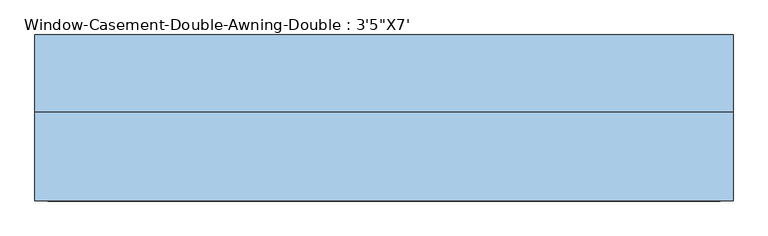
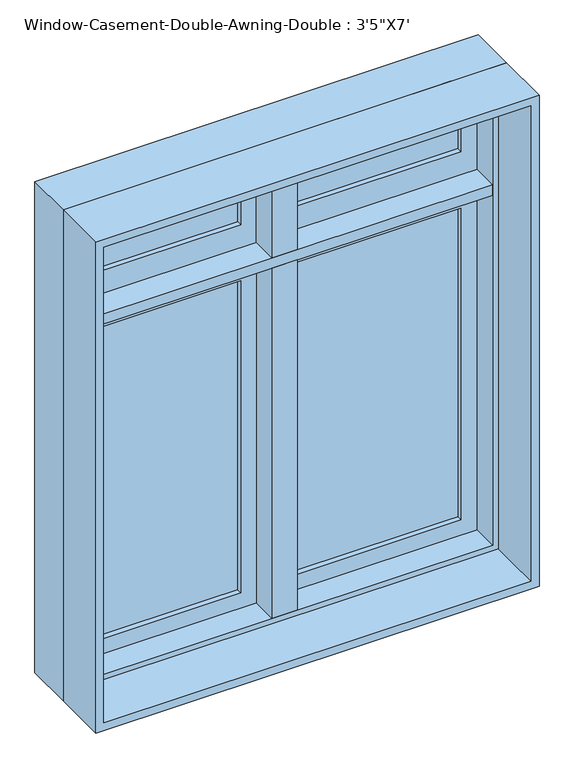
"""IFC4 building model written with IfcOpenShell, lengths in millimetres: window geometry."""

from ifc_helpers import new_model, si_unit, frame, origin, place, context, project, spatial, polyline, outline, extrude, faceted_brep, source, transform, mapped, element, save


def window_35f3c129(model_context):
    return source(origin(), model_context, "Body", "SolidModel", [
        faceted_brep([(488.95, 82.55, 2101.85), (488.95, 19.05, 2101.85), (-488.95, 19.05, 2101.85), (-488.95, 82.55, 2101.85), (508.0, 133.35, 2120.9), (508.0, 82.55, 2120.9), (-508.0, 82.55, 2120.9), (-508.0, 133.35, 2120.9), (520.7, 19.05, 2133.6), (520.7, 133.35, 2133.6), (-520.7, 133.35, 2133.6), (-520.7, 19.05, 2133.6), (-488.95, 19.05, 946.15), (-488.95, 82.55, 946.15), (-508.0, 82.55, 927.1), (-508.0, 133.35, 927.1), (-520.7, 133.35, 914.4), (-520.7, 19.05, 914.4), (488.95, 19.05, 946.15), (488.95, 82.55, 946.15), (508.0, 82.55, 927.1), (508.0, 133.35, 927.1), (520.7, 133.35, 914.4), (520.7, 19.05, 914.4)], [[[0, 1, 2, 3]], [[4, 5, 6, 7]], [[8, 9, 10, 11]], [[3, 2, 12, 13]], [[7, 6, 14, 15]], [[11, 10, 16, 17]], [[13, 12, 18, 19]], [[15, 14, 20, 21]], [[17, 16, 22, 23]], [[11, 17, 23, 8], [1, 18, 12, 2]], [[19, 18, 1, 0]], [[5, 20, 14, 6], [3, 13, 19, 0]], [[21, 20, 5, 4]], [[23, 22, 9, 8]], [[9, 22, 16, 10], [7, 15, 21, 4]]]),
        extrude(outline(polyline([(2133.6, -520.7), (914.4, -520.7), (914.4, 520.7), (2133.6, 520.7), (2133.6, -520.7)]), holes=[polyline([(2114.55, 501.65), (933.45, 501.65), (933.45, -501.65), (2114.55, -501.65), (2114.55, 501.65)])]), frame((0.0, -114.3, 0.0), z_axis=(0.0, 1.0, 0.0), x_axis=(0.0, 0.0, 1.0)), (0.0, 0.0, 1.0), 133.35),
        extrude(outline(polyline([(927.1, 508.0), (1816.1, 508.0), (1816.1, 9.525), (927.1, 9.525), (927.1, 508.0)]), holes=[polyline([(984.25, 66.675), (1758.95, 66.675), (1758.95, 450.85), (984.25, 450.85), (984.25, 66.675)])]), frame((0.0, 82.55, 0.0), z_axis=(0.0, 1.0, 0.0), x_axis=(0.0, 0.0, 1.0)), (0.0, 0.0, 1.0), 44.45),
        extrude(outline(polyline([(1816.1, -508.0), (927.1, -508.0), (927.1, -9.525), (1816.1, -9.525), (1816.1, -508.0)]), holes=[polyline([(1758.95, -66.675), (984.25, -66.675), (984.25, -450.85), (1758.95, -450.85), (1758.95, -66.675)])]), frame((0.0, 82.55, 0.0), z_axis=(0.0, 1.0, 0.0), x_axis=(0.0, 0.0, 1.0)), (0.0, 0.0, 1.0), 44.45),
        extrude(outline(polyline([(450.85, 114.3), (450.85, 107.95), (66.675, 107.95), (66.675, 114.3), (450.85, 114.3)])), frame((0.0, 0.0, 984.25), z_axis=(0.0, 0.0, 1.0), x_axis=(1.0, 0.0, 0.0)), (0.0, 0.0, 1.0), 774.7),
        extrude(outline(polyline([(66.675, 95.25), (66.675, 101.6), (450.85, 101.6), (450.85, 95.25), (66.675, 95.25)])), frame((0.0, 0.0, 984.25), z_axis=(0.0, 0.0, 1.0), x_axis=(1.0, 0.0, 0.0)), (0.0, 0.0, 1.0), 774.7),
        extrude(outline(polyline([(-66.675, 114.3), (-66.675, 107.95), (-450.85, 107.95), (-450.85, 114.3), (-66.675, 114.3)])), frame((0.0, 0.0, 984.25), z_axis=(0.0, 0.0, 1.0), x_axis=(1.0, 0.0, 0.0)), (0.0, 0.0, 1.0), 774.7),
        extrude(outline(polyline([(-450.85, 95.25), (-450.85, 101.6), (-66.675, 101.6), (-66.675, 95.25), (-450.85, 95.25)])), frame((0.0, 0.0, 984.25), z_axis=(0.0, 0.0, 1.0), x_axis=(1.0, 0.0, 0.0)), (0.0, 0.0, 1.0), 774.7),
        faceted_brep([(9.525, 133.35, 1816.1), (-9.525, 133.35, 1816.1), (-9.525, 82.55, 1816.1), (-30.1625, 82.55, 1816.1), (-30.1625, 19.05, 1816.1), (30.1625, 19.05, 1816.1), (30.1625, 82.55, 1816.1), (9.525, 82.55, 1816.1), (9.525, 133.35, 927.1), (9.525, 82.55, 927.1), (-9.525, 82.55, 927.1), (-9.525, 133.35, 927.1), (-9.525, 82.55, 946.15), (-30.1625, 82.55, 946.15), (-30.1625, 19.05, 946.15), (30.1625, 19.05, 946.15), (30.1625, 82.55, 946.15), (9.525, 82.55, 946.15)], [[[0, 1, 2, 3, 4, 5, 6, 7]], [[8, 9, 10, 11]], [[1, 0, 8, 11]], [[2, 1, 11, 10, 12]], [[3, 2, 12, 13]], [[4, 3, 13, 14]], [[5, 4, 14, 15]], [[6, 5, 15, 16]], [[7, 6, 16, 17]], [[0, 7, 17, 9, 8]], [[17, 12, 10, 9]], [[12, 17, 16, 15, 14, 13]]]),
        extrude(outline(polyline([(-66.675, 114.3), (-66.675, 107.95), (-450.85, 107.95), (-450.85, 114.3), (-66.675, 114.3)])), frame((0.0, 0.0, 1898.65), z_axis=(0.0, 0.0, 1.0), x_axis=(1.0, 0.0, 0.0)), (0.0, 0.0, 1.0), 165.1),
        extrude(outline(polyline([(-450.85, 95.25), (-450.85, 101.6), (-66.675, 101.6), (-66.675, 95.25), (-450.85, 95.25)])), frame((0.0, 0.0, 1898.65), z_axis=(0.0, 0.0, 1.0), x_axis=(1.0, 0.0, 0.0)), (0.0, 0.0, 1.0), 165.1),
        extrude(outline(polyline([(508.0, 133.35), (508.0, 82.55), (488.95, 82.55), (488.95, 19.05), (-488.95, 19.05), (-488.95, 82.55), (-508.0, 82.55), (-508.0, 133.35), (508.0, 133.35)])), frame((0.0, 0.0, 1816.1), z_axis=(0.0, 0.0, 1.0), x_axis=(1.0, 0.0, 0.0)), (0.0, 0.0, 1.0), 25.4),
        faceted_brep([(9.525, 82.55, 2120.9), (9.525, 133.35, 2120.9), (-9.525, 133.35, 2120.9), (-9.525, 82.55, 2120.9), (-9.525, 82.55, 1841.5), (-9.525, 133.35, 1841.5), (9.525, 133.35, 1841.5), (9.525, 82.55, 1841.5), (30.1625, 82.55, 1841.5), (30.1625, 19.05, 1841.5), (-30.1625, 19.05, 1841.5), (-30.1625, 82.55, 1841.5), (-30.1625, 82.55, 2101.85), (-9.525, 82.55, 2101.85), (-30.1625, 19.05, 2101.85), (30.1625, 19.05, 2101.85), (30.1625, 82.55, 2101.85), (9.525, 82.55, 2101.85)], [[[0, 1, 2, 3]], [[4, 5, 6, 7, 8, 9, 10, 11]], [[4, 11, 12, 13]], [[11, 10, 14, 12]], [[10, 9, 15, 14]], [[9, 8, 16, 15]], [[8, 7, 17, 16]], [[1, 0, 17, 7, 6]], [[2, 1, 6, 5]], [[3, 2, 5, 4, 13]], [[17, 13, 12, 14, 15, 16]], [[13, 17, 0, 3]]]),
        extrude(outline(polyline([(2120.9, 9.525), (1841.5, 9.525), (1841.5, 508.0), (2120.9, 508.0), (2120.9, 9.525)]), holes=[polyline([(2063.75, 450.85), (1898.65, 450.85), (1898.65, 66.675), (2063.75, 66.675), (2063.75, 450.85)])]), frame((0.0, 82.55, 0.0), z_axis=(0.0, 1.0, 0.0), x_axis=(0.0, 0.0, 1.0)), (0.0, 0.0, 1.0), 44.45),
        extrude(outline(polyline([(1841.5, -9.525), (2120.9, -9.525), (2120.9, -508.0), (1841.5, -508.0), (1841.5, -9.525)]), holes=[polyline([(1898.65, -450.85), (2063.75, -450.85), (2063.75, -66.675), (1898.65, -66.675), (1898.65, -450.85)])]), frame((0.0, 82.55, 0.0), z_axis=(0.0, 1.0, 0.0), x_axis=(0.0, 0.0, 1.0)), (0.0, 0.0, 1.0), 44.45),
        extrude(outline(polyline([(66.675, 114.3), (450.85, 114.3), (450.85, 107.95), (66.675, 107.95), (66.675, 114.3)])), frame((0.0, 0.0, 1898.65), z_axis=(0.0, 0.0, 1.0), x_axis=(1.0, 0.0, 0.0)), (0.0, 0.0, 1.0), 165.1),
        extrude(outline(polyline([(450.85, 95.25), (66.675, 95.25), (66.675, 101.6), (450.85, 101.6), (450.85, 95.25)])), frame((0.0, 0.0, 1898.65), z_axis=(0.0, 0.0, 1.0), x_axis=(1.0, 0.0, 0.0)), (0.0, 0.0, 1.0), 165.1),
    ])


if __name__ == "__main__":
    model = new_model("IFC4")
    model_context = context("Model", 3, world=origin())
    ifc_project = project(units=[si_unit("LENGTHUNIT", "METRE", prefix="MILLI")], contexts=[model_context])
    site = spatial("IfcSite", under=ifc_project)
    building = spatial("IfcBuilding", under=site)
    placement = place(None, origin())
    window_shape = window_35f3c129(model_context)
    element("IfcWindow", 1, ObjectType="Window-Casement-Double-Awning-Double : 3'5\"X7'", at=placement, inside=building, context=model_context, shape_type="MappedRepresentation", body=[
        mapped(window_shape, transform((0.0, 0.0, 0.0), x_axis=(1.0, 0.0, 0.0), y_axis=(0.0, 1.0, 0.0), z_axis=(0.0, 0.0, 1.0))),
    ])
    save(model, "model.ifc")

# Revit data of these elements
# Type "Window-Casement-Double-Awning-Double : 3'5\"X7'"
#   Type Mark = "22"
#   Fire Rating = "0.5h"
#   Assembly Code = "B2020100"
#   Analytic Construction = "Double glazing - domestic"
#   Window Inset [instance default] = 0' - 0"
#   Wall Thickness [instance default] = 0' - 6"
#   Interior Wall Closure [instance default] = 0' - 2 1/4"
#   Half Width = 1' - 8 1/2"
#   Visual Light Transmittance = 0.81
#   Transom Height = 1' - 0"
#   Thermal Resistance (R) = 1.8146 (h·ft²·°F)/BTU
#   Solar Heat Gain Coefficient = 0.76
#   Rough Width = 3' - 5 1/2"
#   Rough Height = 4' - 0 1/2"
#   Open Window Height = 3' - 0"
#   Frame Extension [instance default] = 0' - 0 1/4"
#   Height = 4' - 0"
#   Heat Transfer Coefficient (U) = 0.5511 BTU/(h·ft²·°F)
#   Exterior Wall Closure [instance default] = 0' - 1 1/4"
#   Extension Jamb [instance default] = 0' - 2 1/4"
#   Default Sill Height = 3' - 0"
#   Width = 3' - 5"
#   Top Muntin Visibility = yes
#   Bottom Muntin Visibility = yes
#   Interior Trim Visibility [instance default] = yes
#   Exterior Trim Visibility [instance default] = yes
#   Extension Jamb Visibility [instance default] = yes
#   Interior Trim Material = Wood - Stained
#   Muntin Pattern = Muntin Pattern_2x2 : Muntin Pattern_2x2
#   Interior Trim = Trim-Window-Interior-Flat : Picture Frame
#   Interior Frame Material = Wood - Stained
#   Glass Panel Material = Glass
#   Exterior Trim Material = Clad - White
#   Exterior Trim = Trim-Window-Exterior-Flat : with Sill
#   Exterior Frame Material = Clad - White
#   Wall Closure = (empty or 0)
# Element 1 (IfcWindow, "Window-Casement-Double-Awning-Double : 3'5\"X7'")
#   Wall Thickness = 0' - 9"
#   Extension Jamb = 0' - 5 1/4"
#   Materials on its faces: "Wood - Stained", "Glass", "Clad - White"
# Materials
#   "Wood - Stained": class "Wood", colour RGB 224 178 126, transparency 0, Cost = 0
#   "Glass": class "Glass", colour RGB 0 128 192, transparency 0.75, Description = "Soda Lime Glass", Cost = 0
#   "Clad - White": class "Wood", colour RGB 242 242 238, transparency 0, Cost = 0
